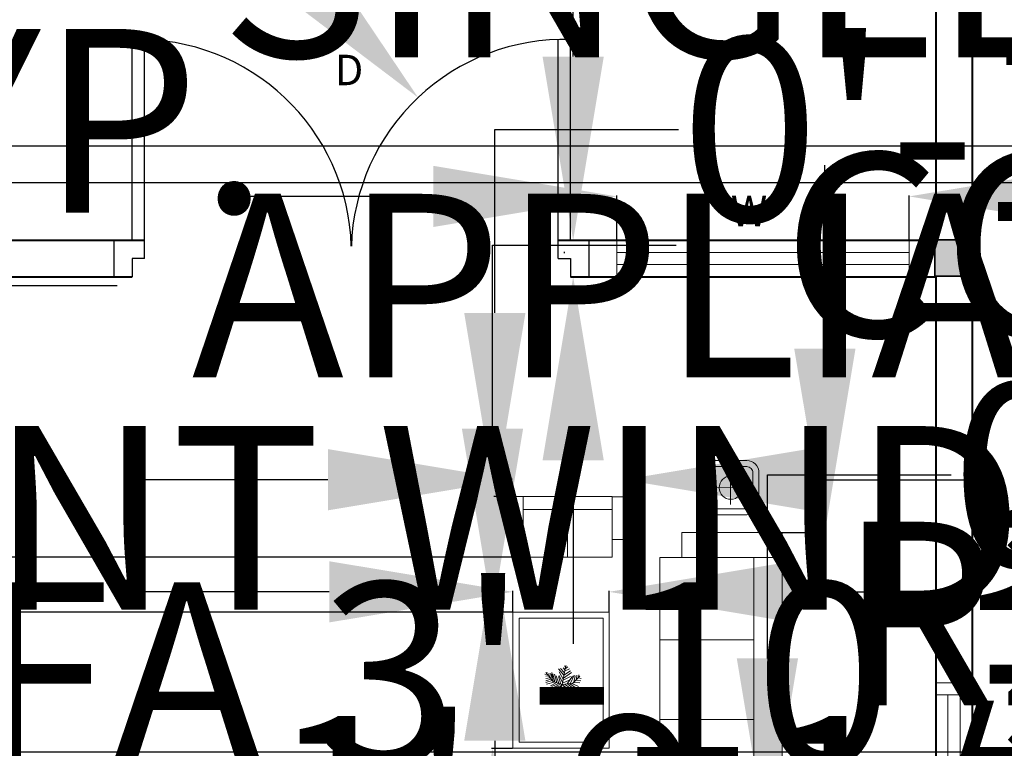
# Model space of a CAD drawing. Units: inches. Extents: x 7323 to 9737, y 2037 to 3322.
# Tile 5 of 19: x 8759 to 8921, y 2420 to 2540. Entities that reach past the tile are written whole.
import ezdxf

# ---------------------------------------------------------------- set-up
doc = ezdxf.new("R2010")
doc.units = ezdxf.units.IN
doc.header["$MEASUREMENT"] = 0
for name, color, linetype, lineweight in [('A-ANNO-DIMS', 2, 'Continuous', 18), ('A-ANNO-TEXT', 7, 'Continuous', 25), ('A-COLS', 1, 'Continuous', 35), ('A-DOOR', 4, 'Continuous', 25), ('A-FURN', 8, 'Continuous', 18), ('A-GLAZ', 4, 'Continuous', 18), ('A-WALL', 7, 'Continuous', 40)]:
    doc.layers.add(name, color=color, linetype=linetype, lineweight=lineweight)
doc.layers.add('A-COLS-PATT', color=18, linetype='Continuous', lineweight=13, true_color=0x000000)
doc.styles.get("Standard").update_dxf_attribs({"font": 'arial.ttf'})
doc.dimstyles.get("Standard").update_dxf_attribs({"dimtxt": 30.18, "dimasz": 30.18, "dimexe": 0.18, "dimexo": 0.0625, "dimgap": 0.09, "dimtad": 0, "dimtih": 1, "dimtoh": 1, "dimdec": 0, "dimzin": 0, "dimdsep": 46, "dimlunit": 3, "dimtxsty": 'Standard', "dimcen": 0.09, "dimadec": 0, "dimazin": 0, "dimtfac": 1, "dimtdec": 0, "dimtofl": 0, "dimtmove": 0, "dimatfit": 3, "dimfxl": 1, "dimtolj": 1, "dimtzin": 0, "dimarcsym": 0})

# ---------------------------------------------------------------- blocks, each defined once
blk = doc.blocks.new('*U4')
for p, q in [((-3.665, 19.273), (-27.574, 35.527)), ((-5.114, 28.097), (-24.676, 40.636)), ((-7.288, 39.707), (-21.778, 46.673)), ((-8.737, 47.138), (-17.069, 52.711)), ((-10.186, 53.64), (-13.084, 55.962)), ((0, 0), (-10.5, 57)), ((-9.099, 51.782), (-6.563, 55.962)), ((-7.65, 43.423), (-2.578, 49.46)), ((-5.839, 35.992), (4.667, 48.067)), ((-5.114, 27.632), (10.463, 46.673)), ((-2.941, 16.486), (8.652, 37.85)), ((16.259, 5.805), (23.142, 31.348)), ((22.055, 7.198), (27.489, 32.277)), ((27, 9), (48, 36)), ((27.127, 9.056), (31.112, 35.992)), ((31.836, 30.883), (32.561, 16.486)), ((35.096, 32.741), (37.27, 22.524)), ((38.719, 34.134), (41.979, 28.561)), ((43.791, 29.954), (51.036, 30.883)), ((44.153, 36.456), (45.239, 32.741)), ((-47.498, 19.737), (-55.83, 18.344)), ((-40.615, 13.7), (-55.105, 10.913)), ((-31.5, 4.5), (-52.5, 25.5)), ((-33.37, 6.269), (-52.207, 5.34)), ((-48.585, 21.131), (-49.309, 29.026)), ((-28.299, 3.483), (-47.86, -5.805)), ((-43.513, 28.561), (-42.427, 15.558)), ((-38.442, 26.239), (-34.819, 7.663)), ((-21.416, 3.018), (-38.079, -8.128)), ((-35.544, 28.097), (-24.314, 3.947)), ((0, 0), (-31.5, 4.5)), ((-14.533, 2.09), (-30.834, 25.31)), ((-15.982, 2.09), (-30.11, -9.521)), ((-24.314, 23.917), (-2.941, 13.7)), ((0, 0), (-22.5, -19.5)), ((-6.563, 1.161), (-21.416, -8.128)), ((-20.691, 13.7), (-1.129, 4.876)), ((-1.129, 6.734), (9.014, 26.704)), ((0, 0), (27, 9)), ((0, 0), (18, -22.5)), ((3.942, 1.625), (11.187, 24.381)), ((6.478, 1.625), (26.04, -8.592)), ((10.101, 3.483), (17.708, 26.239)), ((11.187, 3.483), (30.749, -5.805)), ((18.07, 5.805), (35.096, -3.483)), ((24.229, 7.663), (46.688, 1.625)), ((29.662, 12.307), (48.137, 6.269)), ((33.285, 16.486), (48.862, 10.913)), ((36.183, 19.737), (48.137, 17.88)), ((40.53, 25.775), (48.862, 24.846)), ((-17.431, -15.094), (-42.789, -18.809)), ((-28.299, -29.026), (-42.789, -31.348)), ((-24.314, -21.596), (-42.427, -22.06)), ((-26.849, -26.24), (-40.253, -25.775)), ((-22.5, -19.5), (-37.5, -45)), ((-15.257, -12.772), (-30.11, -12.772)), ((-25.038, -23.918), (-22.865, -45.281)), ((-20.691, -18.345), (-17.793, -44.352)), ((-6.563, -5.805), (-19.967, -9.985)), ((-17.069, -15.094), (-12.721, -40.172)), ((-13.446, -11.378), (-8.737, -32.741)), ((-9.461, -8.592), (-6.201, -23.453)), ((-4.752, -3.483), (-3.665, -14.629)), ((2.493, -3.019), (-1.491, -20.202)), ((1.769, -2.555), (24.229, -9.521)), ((5.029, -6.27), (2.131, -25.775)), ((9.014, -11.378), (3.58, -35.992)), ((14.085, -16.951), (6.478, -40.172)), ((7.565, -9.056), (32.198, -14.629)), ((18.07, -22.524), (8.289, -45.745)), ((12.274, -15.094), (36.907, -18.809)), ((16.259, -19.738), (36.183, -22.989)), ((18, -22.5), (27, -52.5)), ((18.433, -22.524), (40.53, -29.026)), ((19.157, -25.311), (38.719, -33.206)), ((-30.834, -34.135), (-42.427, -35.528)), ((-34.457, -39.708), (-40.978, -42.494)), ((-32.646, -36.921), (-31.921, -44.352)), ((-29.023, -30.884), (-27.936, -43.887)), ((20.244, -30.419), (15.897, -44.816)), ((22.78, -37.85), (19.519, -48.532)), ((21.331, -32.741), (39.081, -40.636)), ((22.78, -38.314), (34.372, -44.816)), ((24.591, -45.745), (23.142, -50.854)), ((24.591, -43.423), (30.749, -47.603)), ((26.764, -49.925), (28.213, -50.854))]:
    blk.add_line(p, q)
blk = doc.blocks.new('DOOR-PAIR-72')
for p, q in [((3, 6), (3, 39)), ((5, 3), (5, 39)), ((73, 3), (73, 39)), ((75, 6), (75, 39)), ((0, 6), (0, 0)), ((38.96, 6), (39.04, 6)), ((39, 6), (39, 5)), ((78, 6), (78, 0)), ((3, 3), (3, 0)), ((5, 3), (3, 3)), ((73, 3), (75, 3)), ((75, 3), (75, 0))]:
    blk.add_line(p, q)
for centre, start, end in [((4, 4), 1.6366, 91.6366), ((74, 4), 88.3634, 178.3634)]:
    blk.add_arc(centre, 35.01, start, end)
blk = doc.blocks.new('WIN-48')
for p, q in [((0, 0), (0, 6)), ((2, 0), (2, 6)), ((50, 0), (50, 6)), ((52, 0), (52, 6)), ((2, 4), (50, 4)), ((2, 2), (50, 2))]:
    blk.add_line(p, q)
blk = doc.blocks.new('WIN-48-SINGLE-JAMB')
for p, q in [((0, 6), (0, 0)), ((48, 6), (48, 0)), ((0, 4), (48, 4)), ((0, 2), (48, 2))]:
    blk.add_line(p, q)
blk = doc.blocks.new('COFFEE-TABLE')
for points in [[(15.8, 22.37), (15.8, 22.37), (0, 22.37), (0, 22.37), (0, 0), (0, 0), (15.8, 0), (15.8, 0)], [(14.8, 21.37), (1, 21.37), (1, 1), (14.8, 1)]]:
    blk.add_lwpolyline(points, close=True)
blk = doc.blocks.new('SOFA-THREE-SEAT')
for p, q in [((15.45, 29), (0, 29)), ((15.45, 29), (0, 29)), ((15.45, 15.91), (0, 15.91)), ((15.45, 15.91), (0, 15.91))]:
    blk.add_line(p, q)
for points in [[(20.12, 42.5), (20.12, 42.5), (3.63, 42.5), (3.63, 42.5), (3.63, 46.66), (3.63, 46.66), (20.12, 46.66), (20.12, 46.66)], [(20.12, 42.5), (20.12, 42.5), (3.63, 42.5), (3.63, 42.5), (3.63, 46.66), (3.63, 46.66), (20.12, 46.66), (20.12, 46.66)], [(15.45, 42.5), (15.45, 42.5), (20.12, 42.5), (20.12, 42.5), (20.12, 4.16), (20.12, 4.16), (15.45, 4.16), (15.45, 4.16)], [(15.45, 42.5), (15.45, 42.5), (20.12, 42.5), (20.12, 42.5), (20.12, 4.16), (20.12, 4.16), (15.45, 4.16), (15.45, 4.16)], [(20.12, 0), (20.12, 0), (3.63, 0), (3.63, 0), (3.63, 4.16), (3.63, 4.16), (20.12, 4.16), (20.12, 4.16)], [(20.12, 0), (20.12, 0), (3.63, 0), (3.63, 0), (3.63, 4.16), (3.63, 4.16), (20.12, 4.16), (20.12, 4.16)]]:
    blk.add_lwpolyline(points, close=True)
blk.add_lwpolyline([(15.45, 4.16), (15.45, 42.5), (15.45, 42.5), (0, 42.5), (0, 42.5), (0, 3.77), (0, 3.77), (3.63, 3.77)])
blk.add_lwpolyline([(15.45, 4.16), (15.45, 42.5), (15.45, 42.5), (0, 42.5), (0, 42.5), (0, 3.77), (0, 3.77), (3.63, 3.77)])
blk = doc.blocks.new('ARMCHAIR')
blk.add_line((9.19, 7.87), (9.19, 0))
for points in [[(0, 9.98), (0, 9.98), (1.9, 9.98), (1.9, 9.98), (1.9, 2.97), (1.9, 2.97), (0, 2.97), (0, 2.97)], [(16.51, 7.87), (16.51, 7.87), (1.9, 7.87), (1.9, 7.87), (1.9, 9.98), (1.9, 9.98), (16.51, 9.98), (16.51, 9.98)], [(16.51, 9.95), (16.51, 9.95), (18.41, 9.95), (18.41, 9.95), (18.41, 2.94), (18.41, 2.94), (16.51, 2.94), (16.51, 2.94)], [(16.51, 7.87), (16.51, 7.87), (1.88, 7.87), (1.88, 7.87), (1.88, 0), (1.88, 0), (16.51, 0), (16.51, 0)]]:
    blk.add_lwpolyline(points, close=True)
blk = doc.blocks.new('LOUNGE-SIDE-TABLE')
for p, q in [((4.58, 7.04), (4.58, 1.66)), ((7.42, 4.45), (1.67, 4.53))]:
    blk.add_line(p, q)
for points in [[(9.25, 6.91, 0.414214), (7.25, 8.91), (2, 8.91, 0.414214), (0, 6.91), (0, 2, 0.414214), (2, 0), (7.25, 0, 0.414214), (9.25, 2)], [(8.25, 6.91, 0.414214), (7.25, 7.91), (2, 7.91, 0.414214), (1, 6.91), (1, 2, 0.414214), (2, 1), (7.25, 1, 0.414214), (8.25, 2)]]:
    blk.add_lwpolyline(points, format="xyb", close=True)
blk.add_circle((4.63, 4.45), 1.91)
blk = doc.blocks.new('COL-PLAN-6IN')
blk.add_lwpolyline([(0, 6), (0, 6), (6.06, 6), (6.06, 6), (6.06, 0), (6.06, 0), (0, 0), (0, 0)], close=True)
blk = doc.blocks.new('*D39')
at = {"layer": 'A-ANNO-DIMS', "color": 0, "lineweight": -2, "transparency": 16777216}
for p, q in [((8678.12, 2543.2), (8678.12, 2549.21)), ((8717.39, 2543.2), (8717.39, 2549.21)), ((8647.94, 2549.03), (8617.76, 2549.03)), ((8747.57, 2549.03), (8777.75, 2549.03))]:
    blk.add_line(p, q, dxfattribs=at)
at = {"layer": 'A-ANNO-DIMS', "color": 0, "transparency": 16777216}
for points in [[(8647.94, 2554.06), (8647.94, 2544), (8678.12, 2549.03)], [(8747.57, 2554.06), (8747.57, 2544), (8717.39, 2549.03)]]:
    blk.add_solid(points, dxfattribs=at)
at = {"layer": 'Defpoints', "color": 0, "transparency": 16777216}
for p in [(8717.39, 2549.03), (8678.12, 2543.14), (8717.39, 2543.14)]:
    blk.add_point(p, dxfattribs=at)
at = {"layer": 'A-ANNO-DIMS', "color": 0, "transparency": 16777216, "insert": (9057.19, 2549.03), "char_height": 30.18, "attachment_point": 5}
blk.add_mtext('\\A1;SINGLE DOOR 3\'-3 1/2" TYP.', dxfattribs=at)
blk = doc.blocks.new('*D40')
at = {"layer": 'A-ANNO-DIMS', "color": 0, "lineweight": -2, "transparency": 16777216}
for p, q in [((8672.23, 2573.32), (8672.23, 2603.5)), ((8678.06, 2543.14), (8672.05, 2543.14)), ((8678.06, 2503.86), (8672.05, 2503.86)), ((8672.23, 2473.68), (8672.23, 2443.5))]:
    blk.add_line(p, q, dxfattribs=at)
at = {"layer": 'A-ANNO-DIMS', "color": 0, "transparency": 16777216}
for points in [[(8667.2, 2573.32), (8677.26, 2573.32), (8672.23, 2543.14)], [(8667.2, 2473.68), (8677.26, 2473.68), (8672.23, 2503.86)]]:
    blk.add_solid(points, dxfattribs=at)
at = {"layer": 'Defpoints', "color": 0, "transparency": 16777216}
for p in [(8672.23, 2543.14), (8678.12, 2543.14), (8678.12, 2503.86)]:
    blk.add_point(p, dxfattribs=at)
at = {"layer": 'A-ANNO-DIMS', "color": 0, "transparency": 16777216, "insert": (8672.23, 2523.5), "char_height": 30.18, "attachment_point": 5}
blk.add_mtext('\\A1;3\'-3 1/2" TYP.', dxfattribs=at)
blk = doc.blocks.new('*D41')
at = {"layer": 'A-ANNO-DIMS', "color": 0, "lineweight": -2, "transparency": 16777216}
for p, q in [((8661.59, 2428.04), (8661.59, 2458.22)), ((8661.59, 2458.22), (8691.77, 2458.22)), ((8657.46, 2397.86), (8661.77, 2397.86)), ((8657.46, 2369.86), (8661.77, 2369.86)), ((8661.59, 2339.68), (8661.59, 2309.5))]:
    blk.add_line(p, q, dxfattribs=at)
at = {"layer": 'A-ANNO-DIMS', "color": 0, "transparency": 16777216}
for points in [[(8656.56, 2428.04), (8666.62, 2428.04), (8661.59, 2397.86)], [(8656.56, 2339.68), (8666.62, 2339.68), (8661.59, 2369.86)]]:
    blk.add_solid(points, dxfattribs=at)
at = {"layer": 'Defpoints', "color": 0, "transparency": 16777216}
for p in [(8657.39, 2397.86), (8661.59, 2397.86), (8657.39, 2369.86)]:
    blk.add_point(p, dxfattribs=at)
at = {"layer": 'A-ANNO-DIMS', "color": 0, "transparency": 16777216, "insert": (8945.06, 2458.22), "char_height": 30.18, "attachment_point": 5}
blk.add_mtext('\\A1;VENT WINDOW 2\'-4" TYP.', dxfattribs=at)
blk = doc.blocks.new('*D43')
at = {"layer": 'A-ANNO-DIMS', "color": 0, "lineweight": -2, "transparency": 16777216}
for p, q in [((9108.94, 2438.75), (9108.94, 2468.93)), ((9104.01, 2408.57), (9109.12, 2408.57)), ((9104.01, 2375.3), (9109.12, 2375.3)), ((9108.94, 2345.12), (9108.94, 2314.94))]:
    blk.add_line(p, q, dxfattribs=at)
at = {"layer": 'A-ANNO-DIMS', "color": 0, "transparency": 16777216}
for points in [[(9103.91, 2438.75), (9113.97, 2438.75), (9108.94, 2408.57)], [(9103.91, 2345.12), (9113.97, 2345.12), (9108.94, 2375.3)]]:
    blk.add_solid(points, dxfattribs=at)
at = {"layer": 'Defpoints', "color": 0, "transparency": 16777216}
for p in [(9103.95, 2408.57), (9108.94, 2408.57), (9103.95, 2375.3)]:
    blk.add_point(p, dxfattribs=at)
at = {"layer": 'A-ANNO-DIMS', "color": 0, "transparency": 16777216, "insert": (9108.94, 2391.93), "char_height": 30.18, "attachment_point": 5}
blk.add_mtext('\\A1;BATH DOOR 2\'-9 1/2" TYP.', dxfattribs=at)
blk = doc.blocks.new('*D47')
at = {"layer": 'A-ANNO-DIMS', "color": 0, "lineweight": -2, "transparency": 16777216}
for p, q in [((8809.55, 2464.49), (8779.37, 2464.49)), ((8839.73, 2461.79), (8839.73, 2464.67)), ((8858.14, 2461.79), (8858.14, 2464.67)), ((8888.32, 2464.49), (8918.5, 2464.49))]:
    blk.add_line(p, q, dxfattribs=at)
at = {"layer": 'A-ANNO-DIMS', "color": 0, "transparency": 16777216}
for points in [[(8809.55, 2469.52), (8809.55, 2459.46), (8839.73, 2464.49)], [(8888.32, 2469.52), (8888.32, 2459.46), (8858.14, 2464.49)]]:
    blk.add_solid(points, dxfattribs=at)
at = {"layer": 'Defpoints', "color": 0, "transparency": 16777216}
for p in [(8858.14, 2464.49), (8839.73, 2461.73), (8858.14, 2461.73)]:
    blk.add_point(p, dxfattribs=at)
at = {"layer": 'A-ANNO-DIMS', "color": 0, "transparency": 16777216, "insert": (9164.9, 2464.49), "char_height": 30.18, "attachment_point": 5}
blk.add_mtext('\\A1;ARMCHAIR 1\'-6 1/2" TYP.', dxfattribs=at)
blk = doc.blocks.new('*D48')
at = {"layer": 'A-ANNO-DIMS', "color": 0, "lineweight": -2, "transparency": 16777216}
for p, q in [((8836.96, 2491.91), (8836.96, 2522.09)), ((8836.96, 2522.09), (8867.14, 2522.09)), ((8839.66, 2461.73), (8836.78, 2461.73)), ((8839.66, 2451.75), (8836.78, 2451.75)), ((8836.96, 2421.57), (8836.96, 2391.39))]:
    blk.add_line(p, q, dxfattribs=at)
at = {"layer": 'A-ANNO-DIMS', "color": 0, "transparency": 16777216}
for points in [[(8831.93, 2491.91), (8841.99, 2491.91), (8836.96, 2461.73)], [(8831.93, 2421.57), (8841.99, 2421.57), (8836.96, 2451.75)]]:
    blk.add_solid(points, dxfattribs=at)
at = {"layer": 'Defpoints', "color": 0, "transparency": 16777216}
for p in [(8836.96, 2461.73), (8839.73, 2461.73), (8839.73, 2451.75)]:
    blk.add_point(p, dxfattribs=at)
at = {"layer": 'A-ANNO-DIMS', "color": 0, "transparency": 16777216, "insert": (8970.94, 2522.09), "char_height": 30.18, "attachment_point": 5}
blk.add_mtext('\\A1;0\'-10" TYP.', dxfattribs=at)
blk = doc.blocks.new('*D53')
at = {"layer": 'A-ANNO-DIMS', "color": 0, "lineweight": -2, "transparency": 16777216}
for p, q in [((8826.85, 2511.06), (8796.67, 2511.06)), ((8857.03, 2503.93), (8857.03, 2511.24)), ((8905.03, 2503.93), (8905.03, 2511.24)), ((8935.21, 2511.06), (8965.39, 2511.06))]:
    blk.add_line(p, q, dxfattribs=at)
at = {"layer": 'A-ANNO-DIMS', "color": 0, "transparency": 16777216}
for points in [[(8826.85, 2516.09), (8826.85, 2506.03), (8857.03, 2511.06)], [(8935.21, 2516.09), (8935.21, 2506.03), (8905.03, 2511.06)]]:
    blk.add_solid(points, dxfattribs=at)
at = {"layer": 'Defpoints', "color": 0, "transparency": 16777216}
for p in [(8905.03, 2511.06), (8857.03, 2503.86), (8905.03, 2503.86)]:
    blk.add_point(p, dxfattribs=at)
at = {"layer": 'A-ANNO-DIMS', "color": 0, "transparency": 16777216, "insert": (9261.3, 2511.06), "char_height": 30.18, "attachment_point": 5}
blk.add_mtext('\\A1;INTERIOR WINDOW 4\'-0" TYP.', dxfattribs=at)
blk = doc.blocks.new('*D54')
at = {"layer": 'A-ANNO-DIMS', "color": 0, "lineweight": -2, "transparency": 16777216}
for p, q in [((8849.83, 2534.04), (8849.83, 2564.22)), ((8849.83, 2564.22), (8880.01, 2564.22)), ((8856.96, 2503.86), (8849.65, 2503.86)), ((8856.96, 2497.86), (8849.65, 2497.86)), ((8849.83, 2467.68), (8849.83, 2437.5))]:
    blk.add_line(p, q, dxfattribs=at)
at = {"layer": 'A-ANNO-DIMS', "color": 0, "transparency": 16777216}
for points in [[(8844.8, 2534.04), (8854.86, 2534.04), (8849.83, 2503.86)], [(8844.8, 2467.68), (8854.86, 2467.68), (8849.83, 2497.86)]]:
    blk.add_solid(points, dxfattribs=at)
at = {"layer": 'Defpoints', "color": 0, "transparency": 16777216}
for p in [(8849.83, 2503.86), (8857.03, 2503.86), (8857.03, 2497.86)]:
    blk.add_point(p, dxfattribs=at)
at = {"layer": 'A-ANNO-DIMS', "color": 0, "transparency": 16777216, "insert": (8972.08, 2564.22), "char_height": 30.18, "attachment_point": 5}
blk.add_mtext('\\A1;0\'-6" TYP.', dxfattribs=at)
blk = doc.blocks.new('*D63')
at = {"layer": 'A-ANNO-DIMS', "color": 0, "lineweight": -2, "transparency": 16777216}
for p, q in [((8744.72, 2466.22), (8744.72, 2496.4)), ((8744.72, 2496.4), (8774.9, 2496.4)), ((8741.46, 2436.04), (8744.9, 2436.04)), ((8741.46, 2413.86), (8744.9, 2413.86)), ((8744.72, 2383.68), (8744.72, 2353.5))]:
    blk.add_line(p, q, dxfattribs=at)
at = {"layer": 'A-ANNO-DIMS', "color": 0, "transparency": 16777216}
for points in [[(8739.69, 2466.22), (8749.75, 2466.22), (8744.72, 2436.04)], [(8739.69, 2383.68), (8749.75, 2383.68), (8744.72, 2413.86)]]:
    blk.add_solid(points, dxfattribs=at)
at = {"layer": 'Defpoints', "color": 0, "transparency": 16777216}
for p in [(8741.39, 2436.04), (8744.72, 2436.04), (8741.39, 2413.86)]:
    blk.add_point(p, dxfattribs=at)
at = {"layer": 'A-ANNO-DIMS', "color": 0, "transparency": 16777216, "insert": (9003.76, 2496.4), "char_height": 30.18, "attachment_point": 5}
blk.add_mtext('\\A1;APPLIANCE 1\'-10" TYP.', dxfattribs=at)
blk = doc.blocks.new('*D64')
at = {"layer": 'A-ANNO-DIMS', "color": 0, "lineweight": -2, "transparency": 16777216}
for p, q in [((8719.69, 2413.8), (8719.69, 2410.36)), ((8741.39, 2413.8), (8741.39, 2410.36)), ((8689.51, 2410.54), (8659.33, 2410.54)), ((8771.57, 2410.54), (8801.75, 2410.54))]:
    blk.add_line(p, q, dxfattribs=at)
at = {"layer": 'A-ANNO-DIMS', "color": 0, "transparency": 16777216}
for points in [[(8689.51, 2415.57), (8689.51, 2405.51), (8719.69, 2410.54)], [(8771.57, 2415.57), (8771.57, 2405.51), (8741.39, 2410.54)]]:
    blk.add_solid(points, dxfattribs=at)
at = {"layer": 'Defpoints', "color": 0, "transparency": 16777216}
for p in [(8719.69, 2413.86), (8741.39, 2413.86), (8741.39, 2410.54)]:
    blk.add_point(p, dxfattribs=at)
at = {"layer": 'A-ANNO-DIMS', "color": 0, "transparency": 16777216, "insert": (8927.57, 2410.54), "char_height": 30.18, "attachment_point": 5}
blk.add_mtext('\\A1;1\'-9 1/2" TYP.', dxfattribs=at)
blk = doc.blocks.new('*D69')
at = {"layer": 'A-ANNO-DIMS', "color": 0, "lineweight": -2, "transparency": 16777216}
for p, q in [((8836.58, 2472.89), (8836.58, 2503.07)), ((8836.58, 2503.07), (8866.76, 2503.07)), ((8839.88, 2442.71), (8836.4, 2442.71)), ((8839.88, 2420.33), (8836.4, 2420.33)), ((8836.58, 2390.15), (8836.58, 2359.97))]:
    blk.add_line(p, q, dxfattribs=at)
at = {"layer": 'A-ANNO-DIMS', "color": 0, "transparency": 16777216}
for points in [[(8831.55, 2472.89), (8841.61, 2472.89), (8836.58, 2442.71)], [(8831.55, 2390.15), (8841.61, 2390.15), (8836.58, 2420.33)]]:
    blk.add_solid(points, dxfattribs=at)
at = {"layer": 'Defpoints', "color": 0, "transparency": 16777216}
for p in [(8836.58, 2442.71), (8839.94, 2442.71), (8839.94, 2420.33)]:
    blk.add_point(p, dxfattribs=at)
at = {"layer": 'A-ANNO-DIMS', "color": 0, "transparency": 16777216, "insert": (9169.54, 2503.07), "char_height": 30.18, "attachment_point": 5}
blk.add_mtext('\\A1;COFFEE TABLE 1\'-10 1/2" TYP.', dxfattribs=at)
blk = doc.blocks.new('*D70')
at = {"layer": 'A-ANNO-DIMS', "color": 0, "lineweight": -2, "transparency": 16777216}
for p, q in [((8809.76, 2446.06), (8779.58, 2446.06)), ((8839.94, 2442.77), (8839.94, 2446.24)), ((8855.74, 2442.77), (8855.74, 2446.24)), ((8885.92, 2446.06), (8916.1, 2446.06))]:
    blk.add_line(p, q, dxfattribs=at)
at = {"layer": 'A-ANNO-DIMS', "color": 0, "transparency": 16777216}
for points in [[(8809.76, 2451.09), (8809.76, 2441.03), (8839.94, 2446.06)], [(8885.92, 2451.09), (8885.92, 2441.03), (8855.74, 2446.06)]]:
    blk.add_solid(points, dxfattribs=at)
at = {"layer": 'Defpoints', "color": 0, "transparency": 16777216}
for p in [(8855.74, 2446.06), (8839.94, 2442.71), (8855.74, 2442.71)]:
    blk.add_point(p, dxfattribs=at)
at = {"layer": 'A-ANNO-DIMS', "color": 0, "transparency": 16777216, "insert": (9006.75, 2446.06), "char_height": 30.18, "attachment_point": 5}
blk.add_mtext('\\A1;1\'-4" TYP.', dxfattribs=at)
blk = doc.blocks.new('*D71')
at = {"layer": 'A-ANNO-DIMS', "color": 0, "lineweight": -2, "transparency": 16777216}
for p, q in [((8891.18, 2486.02), (8891.18, 2516.2)), ((8884.24, 2455.84), (8891.36, 2455.84)), ((8884.24, 2409.18), (8891.36, 2409.18)), ((8891.18, 2379), (8891.18, 2348.82))]:
    blk.add_line(p, q, dxfattribs=at)
at = {"layer": 'A-ANNO-DIMS', "color": 0, "transparency": 16777216}
for points in [[(8886.15, 2486.02), (8896.21, 2486.02), (8891.18, 2455.84)], [(8886.15, 2379), (8896.21, 2379), (8891.18, 2409.18)]]:
    blk.add_solid(points, dxfattribs=at)
at = {"layer": 'Defpoints', "color": 0, "transparency": 16777216}
for p in [(8884.18, 2455.84), (8891.18, 2455.84), (8884.18, 2409.18)]:
    blk.add_point(p, dxfattribs=at)
at = {"layer": 'A-ANNO-DIMS', "color": 0, "transparency": 16777216, "insert": (8891.18, 2432.51), "char_height": 30.18, "attachment_point": 5}
blk.add_mtext('\\A1;SOFA 3\'-10 1/2" TYP.', dxfattribs=at)
blk = doc.blocks.new('*D72')
at = {"layer": 'A-ANNO-DIMS', "color": 0, "lineweight": -2, "transparency": 16777216}
for p, q in [((8864.06, 2409.12), (8864.06, 2402)), ((8884.18, 2409.12), (8884.18, 2402)), ((8833.88, 2402.18), (8803.7, 2402.18)), ((8914.36, 2402.18), (8944.54, 2402.18))]:
    blk.add_line(p, q, dxfattribs=at)
at = {"layer": 'A-ANNO-DIMS', "color": 0, "transparency": 16777216}
for points in [[(8833.88, 2407.21), (8833.88, 2397.15), (8864.06, 2402.18)], [(8914.36, 2407.21), (8914.36, 2397.15), (8884.18, 2402.18)]]:
    blk.add_solid(points, dxfattribs=at)
at = {"layer": 'Defpoints', "color": 0, "transparency": 16777216}
for p in [(8864.06, 2409.18), (8884.18, 2409.18), (8884.18, 2402.18)]:
    blk.add_point(p, dxfattribs=at)
at = {"layer": 'A-ANNO-DIMS', "color": 0, "transparency": 16777216, "insert": (9035.19, 2402.18), "char_height": 30.18, "attachment_point": 5}
blk.add_mtext('\\A1;1\'-8" TYP.', dxfattribs=at)
blk = doc.blocks.new('*D76')
at = {"layer": 'A-ANNO-DIMS', "color": 0, "lineweight": -2, "transparency": 16777216}
for p, q in [((8657.91, 2322.11), (8657.91, 2352.29)), ((8657.91, 2352.29), (8688.09, 2352.29)), ((8659.75, 2291.93), (8657.73, 2291.93)), ((8659.75, 2282.32), (8657.73, 2282.32)), ((8657.91, 2252.14), (8657.91, 2221.96))]:
    blk.add_line(p, q, dxfattribs=at)
at = {"layer": 'A-ANNO-DIMS', "color": 0, "transparency": 16777216}
for points in [[(8652.88, 2322.11), (8662.94, 2322.11), (8657.91, 2291.93)], [(8652.88, 2252.14), (8662.94, 2252.14), (8657.91, 2282.32)]]:
    blk.add_solid(points, dxfattribs=at)
at = {"layer": 'Defpoints', "color": 0, "transparency": 16777216}
for p in [(8657.91, 2291.93), (8659.81, 2291.93), (8659.81, 2282.32)]:
    blk.add_point(p, dxfattribs=at)
at = {"layer": 'A-ANNO-DIMS', "color": 0, "transparency": 16777216, "insert": (8815.32, 2352.29), "char_height": 30.18, "attachment_point": 5}
blk.add_mtext('\\A1;0\'-9 1/2" TYP.', dxfattribs=at)
blk = doc.blocks.new('*D79')
at = {"layer": 'A-ANNO-DIMS', "color": 0, "lineweight": -2, "transparency": 16777216}
for p, q in [((8871.1, 2395.97), (8871.1, 2394.46)), ((8880.36, 2395.97), (8880.36, 2394.46)), ((8840.92, 2394.64), (8810.74, 2394.64)), ((8910.54, 2394.64), (8940.72, 2394.64))]:
    blk.add_line(p, q, dxfattribs=at)
at = {"layer": 'A-ANNO-DIMS', "color": 0, "transparency": 16777216}
for points in [[(8840.92, 2399.67), (8840.92, 2389.61), (8871.1, 2394.64)], [(8910.54, 2399.67), (8910.54, 2389.61), (8880.36, 2394.64)]]:
    blk.add_solid(points, dxfattribs=at)
at = {"layer": 'Defpoints', "color": 0, "transparency": 16777216}
for p in [(8871.1, 2396.03), (8880.36, 2396.03), (8880.36, 2394.64)]:
    blk.add_point(p, dxfattribs=at)
at = {"layer": 'A-ANNO-DIMS', "color": 0, "transparency": 16777216, "insert": (9195.57, 2394.64), "char_height": 30.18, "attachment_point": 5}
blk.add_mtext('\\A1;SIDE TABLE 0\'-9 1/2" TYP.', dxfattribs=at)
blk = doc.blocks.new('*D80')
at = {"layer": 'A-ANNO-DIMS', "color": 0, "lineweight": -2, "transparency": 16777216}
for p, q in [((8881.74, 2435.12), (8881.74, 2465.3)), ((8881.74, 2465.3), (8911.92, 2465.3)), ((8880.42, 2404.94), (8881.92, 2404.94)), ((8880.42, 2396.03), (8881.92, 2396.03)), ((8881.74, 2365.85), (8881.74, 2335.67))]:
    blk.add_line(p, q, dxfattribs=at)
at = {"layer": 'A-ANNO-DIMS', "color": 0, "transparency": 16777216}
for points in [[(8876.71, 2435.12), (8886.77, 2435.12), (8881.74, 2404.94)], [(8876.71, 2365.85), (8886.77, 2365.85), (8881.74, 2396.03)]]:
    blk.add_solid(points, dxfattribs=at)
at = {"layer": 'Defpoints', "color": 0, "transparency": 16777216}
for p in [(8880.36, 2404.94), (8881.74, 2404.94), (8880.36, 2396.03)]:
    blk.add_point(p, dxfattribs=at)
at = {"layer": 'A-ANNO-DIMS', "color": 0, "transparency": 16777216, "insert": (9003.99, 2465.3), "char_height": 30.18, "attachment_point": 5}
blk.add_mtext('\\A1;0\'-9" TYP.', dxfattribs=at)
blk = doc.blocks.new('*D100')
at = {"layer": 'A-ANNO-DIMS', "color": 0, "lineweight": -2, "transparency": 16777216}
for p, q in [((9007.88, 2687.3), (8587.16, 2687.3)), ((8587.34, 2657.12), (8587.34, 2615.8)), ((8587.34, 2543.49), (8587.34, 2584.8)), ((9008.12, 2513.31), (8587.16, 2513.31))]:
    blk.add_line(p, q, dxfattribs=at)
at = {"layer": 'A-ANNO-DIMS', "color": 0, "transparency": 16777216}
for points in [[(8582.31, 2657.12), (8592.37, 2657.12), (8587.34, 2687.3)], [(8582.31, 2543.49), (8592.37, 2543.49), (8587.34, 2513.31)]]:
    blk.add_solid(points, dxfattribs=at)
at = {"layer": 'Defpoints', "color": 0, "transparency": 16777216}
for p in [(9007.95, 2687.3), (8587.34, 2513.31), (9008.18, 2513.31)]:
    blk.add_point(p, dxfattribs=at)
at = {"layer": 'A-ANNO-DIMS', "color": 0, "transparency": 16777216, "insert": (8587.34, 2600.3), "char_height": 30.18, "attachment_point": 5}
blk.add_mtext('\\A1;14\'-6"', dxfattribs=at)
blk = doc.blocks.new('*D106')
at = {"layer": 'A-ANNO-DIMS', "color": 0, "lineweight": -2, "transparency": 16777216}
for p, q in [((9008.12, 2519.31), (8587.16, 2519.31)), ((8587.34, 2489.13), (8587.34, 2439.14)), ((8587.34, 2357.76), (8587.34, 2407.75)), ((9008.23, 2327.58), (8587.16, 2327.58))]:
    blk.add_line(p, q, dxfattribs=at)
at = {"layer": 'A-ANNO-DIMS', "color": 0, "transparency": 16777216}
for points in [[(8582.31, 2489.13), (8592.37, 2489.13), (8587.34, 2519.31)], [(8582.31, 2357.76), (8592.37, 2357.76), (8587.34, 2327.58)]]:
    blk.add_solid(points, dxfattribs=at)
at = {"layer": 'Defpoints', "color": 0, "transparency": 16777216}
for p in [(8587.34, 2519.31), (9008.18, 2519.31), (9008.29, 2327.58)]:
    blk.add_point(p, dxfattribs=at)
at = {"layer": 'A-ANNO-DIMS', "color": 0, "transparency": 16777216, "insert": (8587.34, 2423.44), "char_height": 30.18, "attachment_point": 5}
blk.add_mtext('\\A1;15\'-11 1/2"', dxfattribs=at)
blk = doc.blocks.new('*D108')
at = {"layer": 'A-ANNO-DIMS', "color": 0, "lineweight": -2, "transparency": 16777216}
for p, q in [((8587.34, 2481.93), (8587.34, 2512.11)), ((8841.54, 2451.75), (8587.16, 2451.75)), ((8839.88, 2442.71), (8587.16, 2442.71)), ((8587.34, 2412.53), (8587.34, 2382.35)), ((8587.34, 2382.35), (8557.16, 2382.35))]:
    blk.add_line(p, q, dxfattribs=at)
at = {"layer": 'A-ANNO-DIMS', "color": 0, "transparency": 16777216}
for points in [[(8582.31, 2481.93), (8592.37, 2481.93), (8587.34, 2451.75)], [(8582.31, 2412.53), (8592.37, 2412.53), (8587.34, 2442.71)]]:
    blk.add_solid(points, dxfattribs=at)
at = {"layer": 'Defpoints', "color": 0, "transparency": 16777216}
for p in [(8841.6, 2451.75), (8587.34, 2442.71), (8839.94, 2442.71)]:
    blk.add_point(p, dxfattribs=at)
at = {"layer": 'A-ANNO-DIMS', "color": 0, "transparency": 16777216, "insert": (8516.96, 2382.35), "char_height": 30.18, "attachment_point": 5}
blk.add_mtext('\\A1;0\'-9"', dxfattribs=at)
blk = doc.blocks.new('*D110')
at = {"layer": 'A-ANNO-DIMS', "color": 0, "lineweight": -2, "transparency": 16777216}
for p, q in [((8587.34, 2449.91), (8587.34, 2480.09)), ((9018.85, 2419.73), (8587.16, 2419.73)), ((9018.85, 2375.3), (8587.16, 2375.3)), ((8587.34, 2345.12), (8587.34, 2314.94))]:
    blk.add_line(p, q, dxfattribs=at)
at = {"layer": 'A-ANNO-DIMS', "color": 0, "transparency": 16777216}
for points in [[(8582.31, 2449.91), (8592.37, 2449.91), (8587.34, 2419.73)], [(8582.31, 2345.12), (8592.37, 2345.12), (8587.34, 2375.3)]]:
    blk.add_solid(points, dxfattribs=at)
at = {"layer": 'Defpoints', "color": 0, "transparency": 16777216}
for p in [(8587.34, 2419.73), (9018.91, 2419.73), (9018.91, 2375.3)]:
    blk.add_point(p, dxfattribs=at)
at = {"layer": 'A-ANNO-DIMS', "color": 0, "transparency": 16777216, "insert": (8587.34, 2397.51), "char_height": 30.18, "attachment_point": 5}
blk.add_mtext('\\A1;3\'-8 1/2"', dxfattribs=at)
blk = doc.blocks.new('*D124')
at = {"layer": 'A-ANNO-DIMS', "color": 0, "lineweight": -2, "transparency": 16777216}
for p, q in [((8752.73, 2571.2), (8782.91, 2571.2)), ((8782.91, 2571.2), (8803.63, 2549.26)), ((8848.3, 2501.86), (8848.48, 2501.86)), ((8848.39, 2501.77), (8848.39, 2501.95))]:
    blk.add_line(p, q, dxfattribs=at)
at = {"layer": 'A-ANNO-DIMS', "color": 0, "transparency": 16777216}
blk.add_solid([(8807.29, 2552.71), (8799.97, 2545.81), (8824.35, 2527.32)], dxfattribs=at)
at = {"layer": 'Defpoints', "color": 0, "transparency": 16777216}
for p in [(8824.35, 2527.32), (8848.39, 2501.86)]:
    blk.add_point(p, dxfattribs=at)
at = {"layer": 'A-ANNO-DIMS', "color": 0, "transparency": 16777216, "insert": (8653.33, 2571.2), "char_height": 30.18, "attachment_point": 5}
blk.add_mtext('\\A1;4X R2\'-11"', dxfattribs=at)
blk = doc.blocks.new('*D126')
at = {"layer": 'A-ANNO-DIMS', "color": 0, "lineweight": -2, "transparency": 16777216}
for p, q in [((9109.28, 2586.63), (9139.46, 2586.63)), ((9139.46, 2586.63), (9160.18, 2564.69)), ((9204.86, 2517.3), (9205.04, 2517.3)), ((9204.95, 2517.21), (9204.95, 2517.39))]:
    blk.add_line(p, q, dxfattribs=at)
at = {"layer": 'A-ANNO-DIMS', "color": 0, "transparency": 16777216}
blk.add_solid([(9163.84, 2568.15), (9156.52, 2561.24), (9180.9, 2542.75)], dxfattribs=at)
at = {"layer": 'Defpoints', "color": 0, "transparency": 16777216}
for p in [(9180.9, 2542.75), (9204.95, 2517.3)]:
    blk.add_point(p, dxfattribs=at)
at = {"layer": 'A-ANNO-DIMS', "color": 0, "transparency": 16777216, "insert": (9009.88, 2586.63), "char_height": 30.18, "attachment_point": 5}
blk.add_mtext('\\A1;4X R2\'-11"', dxfattribs=at)
blk = doc.blocks.new('*D127')
at = {"layer": 'A-ANNO-DIMS', "color": 0, "lineweight": -2, "transparency": 16777216}
for p, q in [((9006.57, 2442.49), (9036.75, 2442.49)), ((9036.75, 2442.49), (9058.09, 2421.15)), ((9099.86, 2379.3), (9100.04, 2379.3)), ((9099.95, 2379.21), (9099.95, 2379.39))]:
    blk.add_line(p, q, dxfattribs=at)
at = {"layer": 'A-ANNO-DIMS', "color": 0, "transparency": 16777216}
blk.add_solid([(9061.64, 2424.71), (9054.53, 2417.6), (9079.43, 2399.81)], dxfattribs=at)
at = {"layer": 'Defpoints', "color": 0, "transparency": 16777216}
for p in [(9079.43, 2399.81), (9099.95, 2379.3)]:
    blk.add_point(p, dxfattribs=at)
at = {"layer": 'A-ANNO-DIMS', "color": 0, "transparency": 16777216, "insert": (8951.92, 2442.49), "char_height": 30.18, "attachment_point": 5}
blk.add_mtext('\\A1;R2\'-5"', dxfattribs=at)

msp = doc.modelspace()

# ---------------------------------------------------------------- hatches: boundary and pattern name
at = {"layer": 'A-COLS-PATT'}
h = msp.add_hatch(color=256, dxfattribs=at)
h.dxf.hatch_style = 1
h.paths.add_polyline_path([(8915.39, 2189.86), (8908.77, 2189.86), (8908.77, 2183.86), (8915.39, 2183.86)])
h.paths.add_polyline_path([(8657.61, 2189.86), (8651.55, 2189.86), (8651.55, 2183.86), (8657.61, 2183.86)])
h.paths.add_polyline_path([(8814.13, 2189.86), (8807.39, 2189.86), (8807.39, 2183.86), (8814.13, 2183.86)])
h.paths.add_polyline_path([(8813.39, 2317.86), (8807.36, 2317.86), (8807.36, 2311.86), (8813.39, 2311.86)])
h.paths.add_polyline_path([(8915.34, 2313.13), (8909.39, 2313.13), (8909.39, 2307.13), (8915.34, 2307.13)])
h.paths.add_polyline_path([(8657.62, 2317.86), (8657.39, 2317.86), (8657.39, 2318.08), (8651.55, 2318.08), (8651.55, 2312.08), (8657.62, 2312.08)])
h.paths.add_polyline_path([(8915.39, 2671.84), (8909.37, 2671.84), (8909.37, 2665.86), (8909.39, 2665.86), (8915.39, 2665.84)])
h.paths.add_polyline_path([(8657.59, 2671.81), (8651.52, 2671.81), (8651.52, 2665.81), (8657.39, 2665.81), (8657.39, 2665.86)])
h.paths.add_polyline_path([(8915.28, 2503.94), (8909.39, 2503.94), (8909.39, 2503.86), (8909.22, 2497.94), (8915.28, 2497.94)])
h.paths.add_polyline_path([(8657.53, 2503.86), (8657.39, 2503.86), (8651.46, 2503.96), (8651.46, 2497.96), (8657.53, 2497.96)])
h.paths.add_polyline_path([(9014.24, 2519.3), (9013.95, 2519.3), (9008.18, 2519.31), (9008.18, 2513.31), (9014.24, 2513.31)])
h.paths.add_polyline_path([(9013.95, 2687.3), (9007.95, 2687.3), (9007.95, 2681.3), (9013.95, 2681.3)])
h.paths.add_polyline_path([(9271.95, 2687.3), (9266.01, 2687.3), (9266.01, 2681.35), (9271.95, 2681.35)])
h.paths.add_polyline_path([(9271.95, 2205.3), (9265.32, 2205.3), (9265.32, 2199.3), (9271.95, 2199.3)])
h.paths.add_polyline_path([(9170.68, 2205.3), (9163.95, 2205.3), (9163.95, 2199.3), (9170.68, 2199.3)])
h.paths.add_polyline_path([(9013.95, 2205.3), (9007.95, 2205.3), (9007.95, 2199.3), (9013.95, 2199.3)])
h.paths.add_polyline_path([(9271.95, 2519.51), (9265.95, 2519.51), (9265.95, 2519.3), (9265.93, 2513.51), (9271.95, 2513.51)])
h.paths.add_polyline_path([(9271.95, 2328.64), (9265.95, 2328.64), (9265.95, 2322.64), (9271.95, 2322.64)])
h.paths.add_polyline_path([(9014.35, 2333.3), (9013.95, 2333.3), (9013.95, 2333.58), (9008.29, 2333.58), (9008.29, 2327.58), (9014.35, 2327.58)])

# ---------------------------------------------------------------- linework, layer by layer
at = {"layer": 'A-WALL'}
for p, q in [((8915.39, 2671.86), (8915.39, 2183.86)), ((8909.39, 2665.86), (8909.39, 2503.86)), ((8717.39, 2503.86), (8779.39, 2503.86)), ((8847.39, 2503.86), (8909.39, 2503.86)), ((8657.39, 2497.86), (8777.39, 2497.86)), ((8849.39, 2497.86), (8909.39, 2497.86)), ((8909.39, 2497.86), (8909.39, 2189.86))]:
    msp.add_line(p, q, dxfattribs=at)

# ---------------------------------------------------------------- block references
at = {"layer": 'A-COLS'}
msp.add_blockref('COL-PLAN-6IN', (8909.22, 2497.94), dxfattribs=at)
at = {"layer": 'A-DOOR'}
msp.add_blockref('DOOR-PAIR-72', (8774.39, 2497.86), dxfattribs=at)
at = {"layer": 'A-FURN'}
for name, p in [('LOUNGE-SIDE-TABLE', (8871.1, 2458.73)), ('ARMCHAIR', (8839.72, 2451.75)), ('SOFA-THREE-SEAT', (8864.06, 2409.18)), ('COFFEE-TABLE', (8839.94, 2420.34))]:
    msp.add_blockref(name, p, dxfattribs=at)
at = {"layer": 'A-FURN', "xscale": -0.0555195490297955, "yscale": 0.0555195490297955, "zscale": 0.0555195490297955}
msp.add_blockref('*U4', (8848.03, 2430.8), dxfattribs=at)
at = {"layer": 'A-GLAZ'}
msp.add_blockref('WIN-48-SINGLE-JAMB', (8857.03, 2497.86), dxfattribs=at)
at = {"layer": 'A-GLAZ', "rotation": 89.99999999999191}
msp.add_blockref('WIN-48', (8915.39, 2379.12), dxfattribs=at)

# ---------------------------------------------------------------- texts
at = {"layer": 'A-ANNO-TEXT', "char_height": 5, "attachment_point": 1}
for s, insert in [('D', (8810.67, 2534.35)), ('W', (8875.73, 2511.16))]:
    msp.add_mtext_dynamic_manual_height_columns(s, width=26.304, gutter_width=1, heights=[0], dxfattribs=dict(at, insert=insert))

# ---------------------------------------------------------------- dimensions: what is measured, and where the dimension line sits
at = {"layer": 'A-ANNO-DIMS'}
for base, p1, p2, picture, middle in [((8587.34, 2513.31), (9007.95, 2687.3), (9008.18, 2513.31), '*D100', (8587.34, 2600.3)), ((8587.34, 2519.31), (9008.29, 2327.58), (9008.18, 2519.31), '*D106', (8587.34, 2423.44)), ((8587.34, 2442.71), (8841.6, 2451.75), (8839.94, 2442.71), '*D108', (8516.96, 2382.35)), ((8587.34, 2419.73), (9018.91, 2375.3), (9018.91, 2419.73), '*D110', (8587.34, 2397.51))]:
    dim = msp.add_linear_dim(base=base, p1=p1, p2=p2, angle=90, dimstyle='Standard', override={"dimdec": 1, "dimlfac": 1, "dimrnd": 0, "dimzin": 1, "dimdsep": 46, "dimlunit": 4, "dimfrac": 2}, dxfattribs=at)
    dim.commit()
    dim.dimension.update_dxf_attribs({"geometry": picture, "text_midpoint": middle})
for base, p1, p2, text, picture, middle in [((8717.39, 2549.03), (8678.12, 2543.14), (8717.39, 2543.14), 'SINGLE DOOR <> TYP.', '*D39', (9057.19, 2549.03)), ((8905.03, 2511.06), (8857.03, 2503.86), (8905.03, 2503.86), 'INTERIOR WINDOW <> TYP.', '*D53', (9261.3, 2511.06)), ((8858.14, 2464.49), (8839.73, 2461.73), (8858.14, 2461.73), 'ARMCHAIR <> TYP.', '*D47', (9164.9, 2464.49)), ((8880.36, 2394.64), (8871.1, 2396.03), (8880.36, 2396.03), 'SIDE TABLE <> TYP.', '*D79', (9195.57, 2394.64)), ((8855.74, 2446.06), (8839.94, 2442.71), (8855.74, 2442.71), '<> TYP.', '*D70', (9006.75, 2446.06)), ((8741.39, 2410.54), (8719.69, 2413.86), (8741.39, 2413.86), '<> TYP.', '*D64', (8927.57, 2410.54)), ((8884.18, 2402.18), (8864.06, 2409.18), (8884.18, 2409.18), '<> TYP.', '*D72', (9035.19, 2402.18))]:
    dim = msp.add_linear_dim(base=base, p1=p1, p2=p2, text=text, dimstyle='Standard', override={"dimdec": 1, "dimlfac": 1, "dimrnd": 0, "dimzin": 1, "dimdsep": 46, "dimlunit": 4, "dimfrac": 2}, dxfattribs=at)
    dim.commit()
    dim.dimension.update_dxf_attribs({"geometry": picture, "text_midpoint": middle})
for center, mpoint, picture, middle in [((9204.95, 2517.3), (9180.9, 2542.75), '*D126', (9009.88, 2586.63)), ((8848.39, 2501.86), (8824.35, 2527.32), '*D124', (8653.33, 2571.2))]:
    dim = msp.add_radius_dim(center=center, mpoint=mpoint, text='4X <>', dimstyle='Standard', override={"dimdec": 1, "dimlfac": 1, "dimrnd": 0, "dimzin": 1, "dimdsep": 46, "dimlunit": 4, "dimfrac": 2}, dxfattribs=at)
    dim.commit()
    dim.dimension.update_dxf_attribs({"geometry": picture, "text_midpoint": middle})
for base, p1, p2, text, picture, middle in [((8836.58, 2442.71), (8839.94, 2420.33), (8839.94, 2442.71), 'COFFEE TABLE <> TYP.', '*D69', (9169.54, 2503.07)), ((8849.83, 2503.86), (8857.03, 2497.86), (8857.03, 2503.86), '<> TYP.', '*D54', (8972.08, 2564.22)), ((8672.23, 2543.14), (8678.12, 2503.86), (8678.12, 2543.14), '<> TYP.', '*D40', (8672.23, 2523.5)), ((8836.96, 2461.73), (8839.73, 2451.75), (8839.73, 2461.73), '<> TYP.', '*D48', (8970.94, 2522.09)), ((8744.72, 2436.04), (8741.39, 2413.86), (8741.39, 2436.04), 'APPLIANCE <> TYP.', '*D63', (9003.76, 2496.4)), ((8661.59, 2397.86), (8657.39, 2369.86), (8657.39, 2397.86), 'VENT WINDOW <> TYP.', '*D41', (8945.06, 2458.22)), ((8891.18, 2455.84), (8884.18, 2409.18), (8884.18, 2455.84), 'SOFA <> TYP.', '*D71', (8891.18, 2432.51)), ((9108.94, 2408.57), (9103.95, 2375.3), (9103.95, 2408.57), 'BATH DOOR <> TYP.', '*D43', (9108.94, 2391.93)), ((8881.74, 2404.94), (8880.36, 2396.03), (8880.36, 2404.94), '<> TYP.', '*D80', (9003.99, 2465.3)), ((8657.91, 2291.93), (8659.81, 2282.32), (8659.81, 2291.93), '<> TYP.', '*D76', (8815.32, 2352.29))]:
    dim = msp.add_linear_dim(base=base, p1=p1, p2=p2, angle=90, text=text, dimstyle='Standard', override={"dimdec": 1, "dimlfac": 1, "dimrnd": 0, "dimzin": 1, "dimdsep": 46, "dimlunit": 4, "dimfrac": 2}, dxfattribs=at)
    dim.commit()
    dim.dimension.update_dxf_attribs({"geometry": picture, "text_midpoint": middle})
dim = msp.add_radius_dim(center=(9099.95, 2379.3), mpoint=(9079.43, 2399.81), dimstyle='Standard', override={"dimdec": 1, "dimlfac": 1, "dimrnd": 0, "dimzin": 1, "dimdsep": 46, "dimlunit": 4, "dimfrac": 2}, dxfattribs=at)
dim.commit()
dim.dimension.update_dxf_attribs({"geometry": '*D127', "text_midpoint": (8951.92, 2442.49)})

doc.saveas('drawing.dxf')
